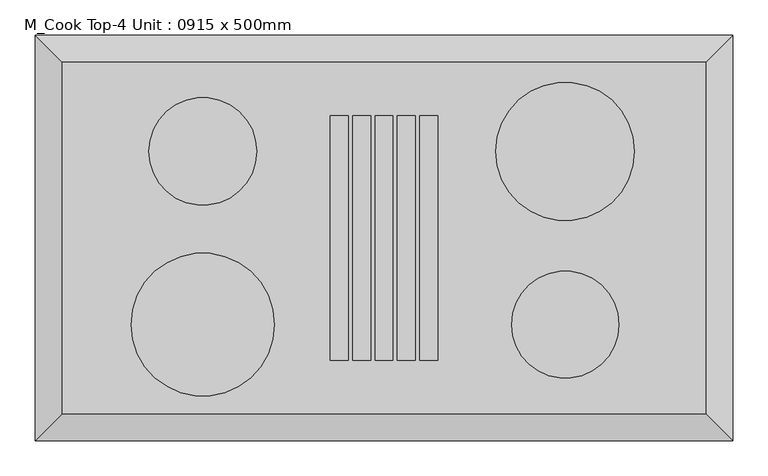
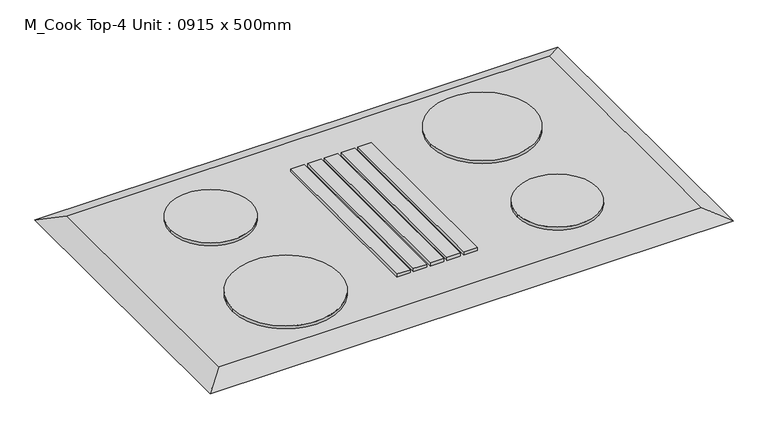
"""IFC4 building model written with IfcOpenShell, lengths in millimetres: proxy geometry, M_Cook Top-4 Unit : 0915 x 500mm."""

from ifc_helpers import new_model, si_unit, point, frame, frame_2d, origin, place, context, project, spatial, polyline, circle_curve, trimmed, segment, composite_curve, outline, extrude, faceted_brep, source, transform, mapped, element, save


def m_cook_top_4_unit_0915_x_500mm_6a9fc197(model_context):
    return source(origin(), model_context, "Body", "SolidModel", [
        faceted_brep([(457.5, 250.0, 918.0), (-457.5, 250.0, 918.0), (-457.5, -250.0, 918.0), (457.5, -250.0, 918.0), (495.6, 288.1, 900.0), (495.6, -288.1, 900.0), (-495.6, -288.1, 900.0), (-495.6, 288.1, 900.0)], [[[0, 1, 2, 3]], [[4, 5, 6, 7]], [[4, 7, 1, 0]], [[7, 6, 2, 1]], [[6, 5, 3, 2]], [[5, 4, 0, 3]]]),
        extrude(outline(composite_curve([segment(trimmed(circle_curve(frame_2d((-257.5, 123.0)), 76.5869489), [point((-180.9130511, 123.0))], [point((-334.0869489, 123.0))], False, "CARTESIAN"), True, "CONTINUOUS"), segment(trimmed(circle_curve(frame_2d((-257.5, 123.0)), 76.5869489), [point((-334.0869489, 123.0))], [point((-180.9130511, 123.0))], False, "CARTESIAN"), True, "CONTINUOUS")], self_intersect=False)), frame((0.0, 0.0, 918.0), z_axis=(0.0, 0.0, 1.0), x_axis=(1.0, 0.0, 0.0)), (0.0, 0.0, 1.0), 6.35),
        extrude(outline(composite_curve([segment(trimmed(circle_curve(frame_2d((257.5, 123.0)), 98.4), [point((355.9, 123.0))], [point((159.1, 123.0))], False, "CARTESIAN"), True, "CONTINUOUS"), segment(trimmed(circle_curve(frame_2d((257.5, 123.0)), 98.4), [point((159.1, 123.0))], [point((355.9, 123.0))], False, "CARTESIAN"), True, "CONTINUOUS")], self_intersect=False)), frame((0.0, 0.0, 918.0), z_axis=(0.0, 0.0, 1.0), x_axis=(1.0, 0.0, 0.0)), (0.0, 0.0, 1.0), 6.35),
        extrude(outline(composite_curve([segment(trimmed(circle_curve(frame_2d((257.5, -123.0)), 76.2), [point((333.7, -123.0))], [point((181.3, -123.0))], False, "CARTESIAN"), True, "CONTINUOUS"), segment(trimmed(circle_curve(frame_2d((257.5, -123.0)), 76.2), [point((181.3, -123.0))], [point((333.7, -123.0))], False, "CARTESIAN"), True, "CONTINUOUS")], self_intersect=False)), frame((0.0, 0.0, 918.0), z_axis=(0.0, 0.0, 1.0), x_axis=(1.0, 0.0, 0.0)), (0.0, 0.0, 1.0), 6.35),
        extrude(outline(polyline([(-50.8, 173.8), (-50.8, -173.8), (-76.2, -173.8), (-76.2, 173.8), (-50.8, 173.8)])), frame((0.0, 0.0, 918.0), z_axis=(0.0, 0.0, 1.0), x_axis=(1.0, 0.0, 0.0)), (0.0, 0.0, 1.0), 6.35),
        extrude(outline(polyline([(-19.05, 173.8), (-19.05, -173.8), (-44.45, -173.8), (-44.45, 173.8), (-19.05, 173.8)])), frame((0.0, 0.0, 918.0), z_axis=(0.0, 0.0, 1.0), x_axis=(1.0, 0.0, 0.0)), (0.0, 0.0, 1.0), 6.35),
        extrude(outline(polyline([(12.7, 173.8), (12.7, -173.8), (-12.7, -173.8), (-12.7, 173.8), (12.7, 173.8)])), frame((0.0, 0.0, 918.0), z_axis=(0.0, 0.0, 1.0), x_axis=(1.0, 0.0, 0.0)), (0.0, 0.0, 1.0), 6.35),
        extrude(outline(polyline([(44.45, 173.8), (44.45, -173.8), (19.05, -173.8), (19.05, 173.8), (44.45, 173.8)])), frame((0.0, 0.0, 918.0), z_axis=(0.0, 0.0, 1.0), x_axis=(1.0, 0.0, 0.0)), (0.0, 0.0, 1.0), 6.35),
        extrude(outline(polyline([(76.2, 173.8), (76.2, -173.8), (50.8, -173.8), (50.8, 173.8), (76.2, 173.8)])), frame((0.0, 0.0, 918.0), z_axis=(0.0, 0.0, 1.0), x_axis=(1.0, 0.0, 0.0)), (0.0, 0.0, 1.0), 6.35),
        extrude(outline(composite_curve([segment(trimmed(circle_curve(frame_2d((-257.5, -123.0)), 101.6), [point((-155.9, -123.0))], [point((-359.1, -123.0))], False, "CARTESIAN"), True, "CONTINUOUS"), segment(trimmed(circle_curve(frame_2d((-257.5, -123.0)), 101.6), [point((-359.1, -123.0))], [point((-155.9, -123.0))], False, "CARTESIAN"), True, "CONTINUOUS")], self_intersect=False)), frame((0.0, 0.0, 918.0), z_axis=(0.0, 0.0, 1.0), x_axis=(1.0, 0.0, 0.0)), (0.0, 0.0, 1.0), 6.35),
    ])


if __name__ == "__main__":
    model = new_model("IFC4")
    model_context = context("Model", 3, world=origin())
    ifc_project = project(units=[si_unit("LENGTHUNIT", "METRE", prefix="MILLI")], contexts=[model_context])
    site = spatial("IfcSite", under=ifc_project)
    building = spatial("IfcBuilding", under=site)
    placement = place(None, origin())
    m_cook_top_4_unit_0915_x_500mm_shape = m_cook_top_4_unit_0915_x_500mm_6a9fc197(model_context)
    element("IfcBuildingElementProxy", 1, Name="M_Cook Top-4 Unit : 0915 x 500mm", ObjectType="M_Cook Top-4 Unit : 0915 x 500mm", at=placement, inside=building, context=model_context, shape_type="MappedRepresentation", body=[
        mapped(m_cook_top_4_unit_0915_x_500mm_shape, transform((0.0, 0.0, 0.0), x_axis=(1.0, 0.0, 0.0), y_axis=(0.0, 1.0, 0.0), z_axis=(0.0, 0.0, 1.0))),
    ])
    save(model, "model.ifc")

# Revit data of these elements
# Type "M_Cook Top-4 Unit : 0915 x 500mm"
#   Counter Height = 900 mm
#   Depth = 500 mm
#   Width = 915 mm
#   Burner Material = Metal - Chrome
#   Cooktop Material = Metal - Steel, Polished
#   Default Elevation = 0
# Element 1 (IfcBuildingElementProxy, "M_Cook Top-4 Unit : 0915 x 500mm")
#   Materials on its faces: "Metal - Chrome", "Metal - Steel, Polished"
# Materials
#   "Metal - Chrome": colour RGB 17 17 17, transparency 0
#   "Metal - Steel, Polished": class "Metal", colour RGB 57 57 57, transparency 0
